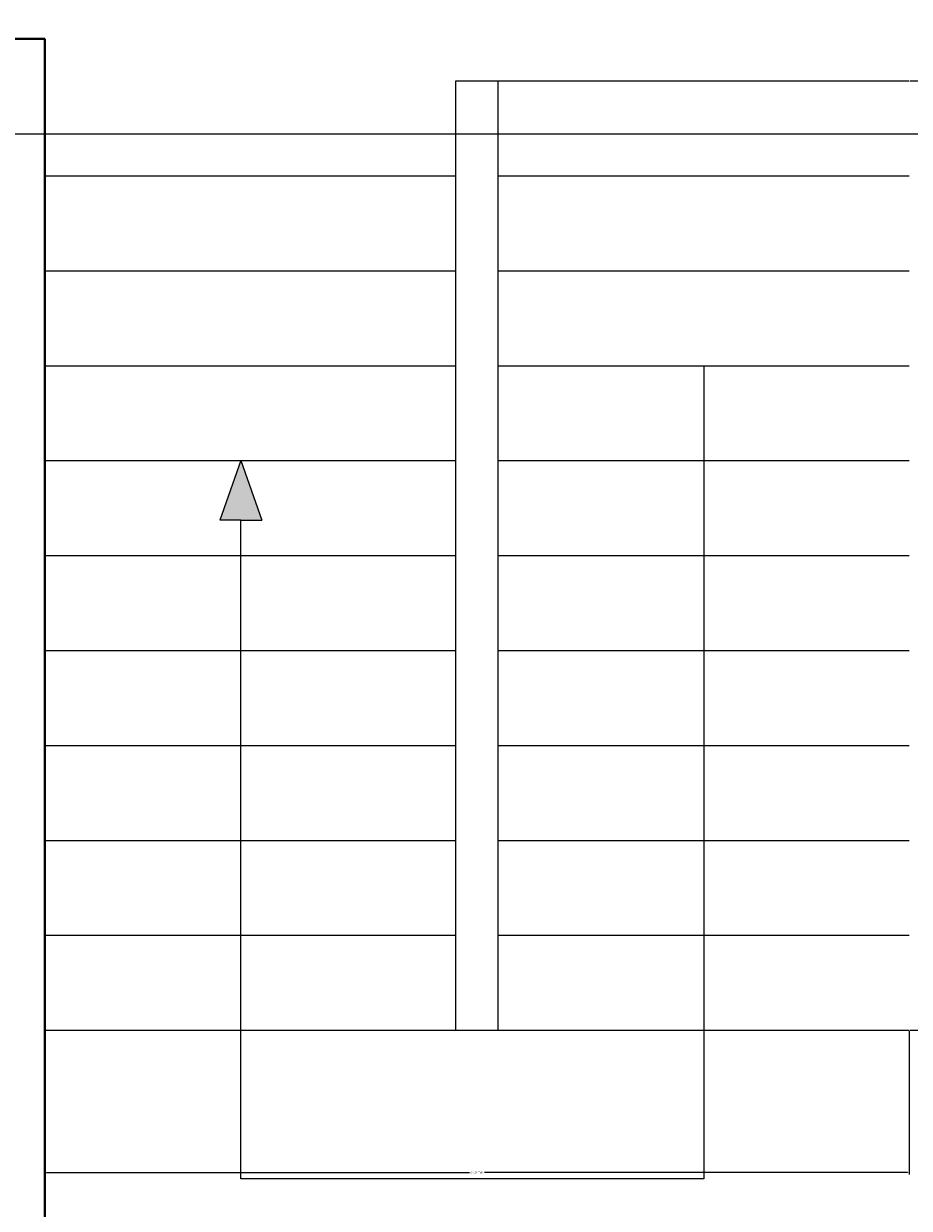
# Model space of a CAD drawing. Units: inches. Extents: x 182 to 1022, y -617 to 111.
# Tile 25 of 33: x 879 to 963, y -507 to -395. Entities that reach past the tile are written whole.
import ezdxf

# ---------------------------------------------------------------- set-up
doc = ezdxf.new("R2010")
doc.units = ezdxf.units.IN
doc.header["$MEASUREMENT"] = 0
for name, color, linetype, lineweight in [('A-ANNO-DIMS', 2, 'Continuous', 18), ('A-ANNO-PATT', 1, 'Continuous', 15), ('A-ANNO-SYMB', 1, 'Continuous', 15), ('A-FLOR-STRS', 1, 'Continuous', 20), ('wall', 1, 'Continuous', 40)]:
    doc.layers.add(name, color=color, linetype=linetype, lineweight=lineweight)
doc.styles.get("Standard").update_dxf_attribs({"font": 'arial.ttf'})
doc.dimstyles.get("Standard").update_dxf_attribs({"dimtxt": 0.18, "dimasz": 0.18, "dimexe": 0.18, "dimexo": 0.0625, "dimgap": 0.09, "dimtad": 0, "dimtih": 1, "dimtoh": 1, "dimdec": 1, "dimzin": 0, "dimdsep": 46, "dimlunit": 4, "dimtxsty": 'Standard', "dimcen": 0.09, "dimadec": 0, "dimazin": 0, "dimtfac": 1, "dimtdec": 1, "dimtofl": 0, "dimtmove": 0, "dimatfit": 3, "dimfxl": 1, "dimtolj": 1, "dimtzin": 0, "dimarcsym": 0})

# ---------------------------------------------------------------- blocks, each defined once
blk = doc.blocks.new('STAIR-DOGLEG')
for p, q in [((39, 0), (39, 90)), ((39, 90), (82, 90)), ((43, 0), (43, 90)), ((0, 81), (39, 81)), ((43, 81), (82, 81)), ((0, 72), (39, 72)), ((43, 72), (82, 72)), ((0, 63), (39, 63)), ((43, 63), (82, 63)), ((0, 54), (39, 54)), ((43, 54), (82, 54)), ((0, 45), (39, 45)), ((43, 45), (82, 45)), ((0, 36), (39, 36)), ((43, 36), (82, 36)), ((0, 27), (39, 27)), ((43, 27), (82, 27)), ((0, 18), (39, 18)), ((43, 18), (82, 18)), ((0, 9), (39, 9)), ((43, 9), (82, 9)), ((0, 0), (82, 0))]:
    blk.add_line(p, q)
blk = doc.blocks.new('*D28')
at = {"layer": 'A-ANNO-DIMS', "color": 0, "lineweight": -2, "transparency": 16777216}
for p, q in [((963.37, -400.37), (976.98, -400.37)), ((976.8, -400.55), (976.8, -445.19)), ((976.8, -490.19), (976.8, -445.56)), ((963.37, -490.37), (976.98, -490.37))]:
    blk.add_line(p, q, dxfattribs=at)
at = {"layer": 'A-ANNO-DIMS', "color": 0, "transparency": 16777216}
for points in [[(976.77, -400.55), (976.83, -400.55), (976.8, -400.37)], [(976.77, -490.19), (976.83, -490.19), (976.8, -490.37)]]:
    blk.add_solid(points, dxfattribs=at)
at = {"layer": 'Defpoints', "color": 0, "transparency": 16777216}
for p in [(963.3, -400.37), (976.8, -400.37), (963.3, -490.37)]:
    blk.add_point(p, dxfattribs=at)
at = {"layer": 'A-ANNO-DIMS', "color": 0, "transparency": 16777216, "insert": (976.8, -445.37), "char_height": 0.18, "attachment_point": 5}
blk.add_mtext('\\A1;STAIR FLIGHTS 7\'-6" TYP.', dxfattribs=at)
blk = doc.blocks.new('*D29')
at = {"layer": 'A-ANNO-DIMS', "color": 0, "lineweight": -2, "transparency": 16777216}
for p, q in [((881.3, -490.44), (881.3, -504.05)), ((963.3, -490.44), (963.3, -504.05)), ((881.48, -503.87), (921.6, -503.87)), ((963.12, -503.87), (923.01, -503.87))]:
    blk.add_line(p, q, dxfattribs=at)
at = {"layer": 'A-ANNO-DIMS', "color": 0, "transparency": 16777216}
for points in [[(881.48, -503.84), (881.48, -503.9), (881.3, -503.87)], [(963.12, -503.84), (963.12, -503.9), (963.3, -503.87)]]:
    blk.add_solid(points, dxfattribs=at)
at = {"layer": 'Defpoints', "color": 0, "transparency": 16777216}
for p in [(881.3, -490.37), (963.3, -490.37), (963.3, -503.87)]:
    blk.add_point(p, dxfattribs=at)
at = {"layer": 'A-ANNO-DIMS', "color": 0, "transparency": 16777216, "insert": (922.3, -503.87), "char_height": 0.18, "attachment_point": 5}
blk.add_mtext('\\A1;6\'-10" TYP.', dxfattribs=at)
blk = doc.blocks.new('*D39')
at = {"layer": 'A-ANNO-DIMS', "color": 0, "lineweight": -2, "transparency": 16777216}
for p, q in [((238.4, -288.54), (1015.28, -288.54)), ((1015.1, -288.72), (1015.1, -346.77)), ((1015.1, -405.19), (1015.1, -347.14)), ((238.43, -405.37), (1015.28, -405.37))]:
    blk.add_line(p, q, dxfattribs=at)
at = {"layer": 'A-ANNO-DIMS', "color": 0, "transparency": 16777216}
for points in [[(1015.07, -288.72), (1015.13, -288.72), (1015.1, -288.54)], [(1015.07, -405.19), (1015.13, -405.19), (1015.1, -405.37)]]:
    blk.add_solid(points, dxfattribs=at)
at = {"layer": 'Defpoints', "color": 0, "transparency": 16777216}
for p in [(238.34, -288.54), (1015.1, -288.54), (238.36, -405.37)]:
    blk.add_point(p, dxfattribs=at)
at = {"layer": 'A-ANNO-DIMS', "color": 0, "transparency": 16777216, "insert": (1015.1, -346.96), "char_height": 0.18, "attachment_point": 5}
blk.add_mtext('\\A1;9\'-9"', dxfattribs=at)

msp = doc.modelspace()

# ---------------------------------------------------------------- hatches: boundary and pattern name
at = {"layer": 'A-ANNO-PATT'}
h = msp.add_hatch(color=256, dxfattribs=at)
h.dxf.hatch_style = 1
h.paths.add_polyline_path([(492.96, -436.37), (490.96, -442.01), (492.96, -442.01), (494.96, -442.01)])
h.paths.add_polyline_path([(899.9, -436.37), (897.9, -442.01), (899.9, -442.01), (901.9, -442.01)])

# ---------------------------------------------------------------- linework, layer by layer
at = {"layer": 'A-ANNO-SYMB'}
for p, q in [((943.8, -427.37), (943.8, -504.45)), ((899.9, -436.37), (897.9, -442.01)), ((899.9, -436.37), (901.9, -442.01)), ((899.9, -442.01), (897.9, -442.01)), ((899.9, -504.45), (899.9, -442.01)), ((899.9, -442.01), (901.9, -442.01)), ((943.8, -504.45), (899.9, -504.45))]:
    msp.add_line(p, q, dxfattribs=at)
at = {"layer": 'wall'}
for p, q in [((681.3, -396.37), (881.3, -396.37)), ((881.3, -396.37), (881.3, -531.37))]:
    msp.add_line(p, q, dxfattribs=at)

# ---------------------------------------------------------------- block references
at = {"layer": 'A-FLOR-STRS'}
msp.add_blockref('STAIR-DOGLEG', (881.3, -490.37), dxfattribs=at)

# ---------------------------------------------------------------- dimensions: what is measured, and where the dimension line sits
at = {"layer": 'A-ANNO-DIMS'}
dim = msp.add_linear_dim(base=(1015.1, -288.54), p1=(238.36, -405.37), p2=(238.34, -288.54), angle=90, dimstyle='Standard', override={"dimdec": 1, "dimlfac": 1, "dimrnd": 0, "dimzin": 1, "dimdsep": 46, "dimlunit": 4, "dimfrac": 2}, dxfattribs=at)
dim.commit()
dim.dimension.update_dxf_attribs({"geometry": '*D39', "text_midpoint": (1015.1, -346.96)})
dim = msp.add_linear_dim(base=(976.8, -400.37), p1=(963.3, -490.37), p2=(963.3, -400.37), angle=90, text='STAIR FLIGHTS <> TYP.', dimstyle='Standard', override={"dimdec": 1, "dimlfac": 1, "dimrnd": 0, "dimzin": 1, "dimdsep": 46, "dimlunit": 4, "dimfrac": 2}, dxfattribs=at)
dim.commit()
dim.dimension.update_dxf_attribs({"geometry": '*D28', "text_midpoint": (976.8, -445.37)})
dim = msp.add_linear_dim(base=(963.3, -503.87), p1=(881.3, -490.37), p2=(963.3, -490.37), text='<> TYP.', dimstyle='Standard', override={"dimdec": 1, "dimlfac": 1, "dimrnd": 0, "dimzin": 1, "dimdsep": 46, "dimlunit": 4, "dimfrac": 2}, dxfattribs=at)
dim.commit()
dim.dimension.update_dxf_attribs({"geometry": '*D29', "text_midpoint": (922.3, -503.87)})

doc.saveas('drawing.dxf')
